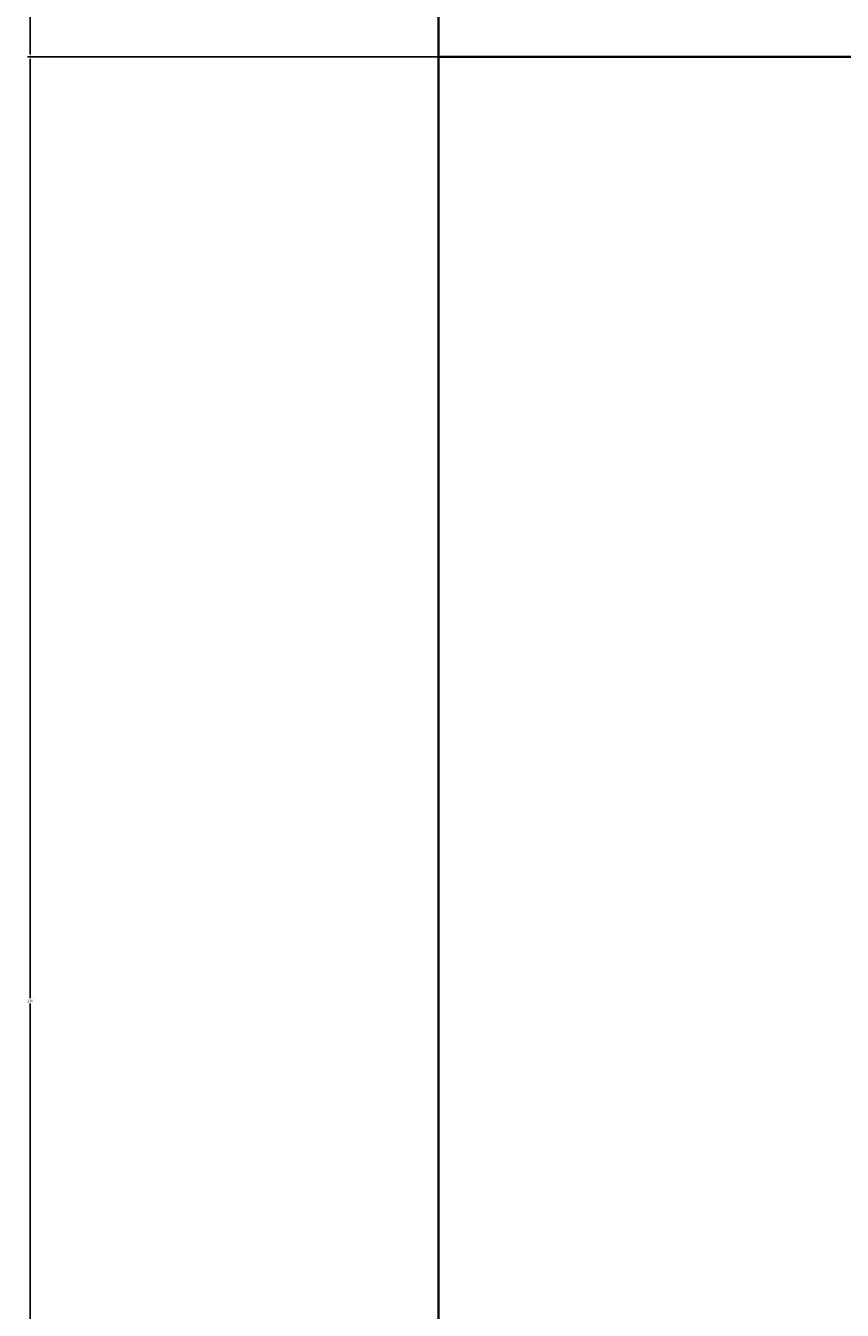
# Model space of a CAD drawing. Units: inches. Extents: x 1911 to 3278, y 2022 to 3108.
# Tile 3 of 13: x 1988 to 2045, y 2178 to 2266. Entities that reach past the tile are written whole.
import ezdxf

# ---------------------------------------------------------------- set-up
doc = ezdxf.new("R2010")
doc.units = ezdxf.units.IN
doc.layers.add('A-ANNO-DIMS', color=2, linetype='Continuous', lineweight=18)
doc.layers.add('A-WALL', color=7, linetype='Continuous', lineweight=35)
doc.styles.get("Standard").update_dxf_attribs({"font": 'arial.ttf'})
doc.dimstyles.get("Standard").update_dxf_attribs({"dimtxt": 0.18, "dimasz": 0.18, "dimexe": 0.18, "dimexo": 0.0625, "dimgap": 0.09, "dimtad": 0, "dimtih": 1, "dimtoh": 1, "dimdec": 4, "dimzin": 0, "dimdsep": 46, "dimtxsty": 'Standard', "dimcen": 0.09, "dimadec": 0, "dimazin": 0, "dimtfac": 1, "dimtdec": 4, "dimtofl": 0, "dimtmove": 0, "dimatfit": 3, "dimfxl": 1, "dimtolj": 1, "dimtzin": 0, "dimarcsym": 0})

# ---------------------------------------------------------------- blocks, each defined once
blk = doc.blocks.new('*D68')
at = {"layer": 'A-ANNO-DIMS', "color": 0, "lineweight": -2, "transparency": 16777216}
for p, q in [((2016.834, 2263.811), (2016.834, 2048.124)), ((2117.834, 2263.811), (2117.834, 2048.124)), ((2017.014, 2048.304), (2067.071, 2048.304)), ((2117.654, 2048.304), (2067.597, 2048.304))]:
    blk.add_line(p, q, dxfattribs=at)
at = {"layer": 'A-ANNO-DIMS', "color": 0, "transparency": 16777216}
for points in [[(2017.014, 2048.334), (2017.014, 2048.274), (2016.834, 2048.304)], [(2117.654, 2048.334), (2117.654, 2048.274), (2117.834, 2048.304)]]:
    blk.add_solid(points, dxfattribs=at)
at = {"layer": 'Defpoints', "color": 0, "transparency": 16777216}
for p in [(2016.834, 2263.873), (2117.834, 2263.873), (2117.834, 2048.304)]:
    blk.add_point(p, dxfattribs=at)
at = {"layer": 'A-ANNO-DIMS', "color": 0, "transparency": 16777216, "insert": (2067.334, 2048.304), "char_height": 0.18, "attachment_point": 5}
blk.add_mtext('\\A1;101', dxfattribs=at)
blk = doc.blocks.new('*D69')
at = {"layer": 'A-ANNO-DIMS', "color": 0, "lineweight": -2, "transparency": 16777216}
for p, q in [((2016.772, 2263.873), (1988.554, 2263.873)), ((1988.734, 2263.693), (1988.734, 2199.055)), ((1988.734, 2134.053), (1988.734, 2198.691)), ((2016.772, 2133.873), (1988.554, 2133.873))]:
    blk.add_line(p, q, dxfattribs=at)
at = {"layer": 'A-ANNO-DIMS', "color": 0, "transparency": 16777216}
for points in [[(1988.704, 2263.693), (1988.764, 2263.693), (1988.734, 2263.873)], [(1988.704, 2134.053), (1988.764, 2134.053), (1988.734, 2133.873)]]:
    blk.add_solid(points, dxfattribs=at)
at = {"layer": 'Defpoints', "color": 0, "transparency": 16777216}
for p in [(2016.834, 2263.873), (1988.734, 2133.873), (2016.834, 2133.873)]:
    blk.add_point(p, dxfattribs=at)
at = {"layer": 'A-ANNO-DIMS', "color": 0, "transparency": 16777216, "insert": (1988.734, 2198.873), "char_height": 0.18, "attachment_point": 5}
blk.add_mtext('\\A1;130', dxfattribs=at)
blk = doc.blocks.new('*D70')
at = {"layer": 'A-ANNO-DIMS', "color": 0, "lineweight": -2, "transparency": 16777216}
for p, q in [((2134.103, 2181.811), (2134.103, 2048.124)), ((2016.834, 2133.811), (2016.834, 2048.124)), ((2017.014, 2048.304), (2075.014, 2048.304)), ((2133.923, 2048.304), (2075.924, 2048.304))]:
    blk.add_line(p, q, dxfattribs=at)
at = {"layer": 'A-ANNO-DIMS', "color": 0, "transparency": 16777216}
for points in [[(2017.014, 2048.334), (2017.014, 2048.274), (2016.834, 2048.304)], [(2133.923, 2048.334), (2133.923, 2048.274), (2134.103, 2048.304)]]:
    blk.add_solid(points, dxfattribs=at)
at = {"layer": 'Defpoints', "color": 0, "transparency": 16777216}
for p in [(2134.103, 2181.873), (2016.834, 2133.873), (2134.103, 2048.304)]:
    blk.add_point(p, dxfattribs=at)
at = {"layer": 'A-ANNO-DIMS', "color": 0, "transparency": 16777216, "insert": (2075.469, 2048.304), "char_height": 0.18, "attachment_point": 5}
blk.add_mtext('\\A1;117.27', dxfattribs=at)
blk = doc.blocks.new('*D72')
at = {"layer": 'A-ANNO-DIMS', "color": 0, "lineweight": -2, "transparency": 16777216}
for p, q in [((2016.772, 2358.3), (1988.554, 2358.3)), ((1988.734, 2358.12), (1988.734, 2311.269)), ((1988.734, 2264.053), (1988.734, 2310.905)), ((2016.772, 2263.873), (1988.554, 2263.873))]:
    blk.add_line(p, q, dxfattribs=at)
at = {"layer": 'A-ANNO-DIMS', "color": 0, "transparency": 16777216}
for points in [[(1988.704, 2358.12), (1988.764, 2358.12), (1988.734, 2358.3)], [(1988.704, 2264.053), (1988.764, 2264.053), (1988.734, 2263.873)]]:
    blk.add_solid(points, dxfattribs=at)
at = {"layer": 'Defpoints', "color": 0, "transparency": 16777216}
for p in [(1988.734, 2358.3), (2016.834, 2358.3), (2016.834, 2263.873)]:
    blk.add_point(p, dxfattribs=at)
at = {"layer": 'A-ANNO-DIMS', "color": 0, "transparency": 16777216, "insert": (1988.734, 2311.087), "char_height": 0.18, "attachment_point": 5}
blk.add_mtext('\\A1;94.43', dxfattribs=at)

msp = doc.modelspace()

# ---------------------------------------------------------------- linework, layer by layer
at = {"layer": 'A-WALL'}
for p, q in [((2016.8344, 2620.8733), (2016.8344, 2133.8733)), ((2016.8344, 2620.8733), (2016.8344, 2133.8733)), ((2016.8344, 2263.8733), (2117.8344, 2263.8733))]:
    msp.add_line(p, q, dxfattribs=at)

# ---------------------------------------------------------------- dimensions: what is measured, and where the dimension line sits
at = {"layer": 'A-ANNO-DIMS'}
for base, p2, override, picture, middle in [((1988.7344, 2358.3003), (2016.8344, 2358.3003), {"dimdec": 2, "dimlfac": 1, "dimrnd": 0, "dimzin": 0, "dimdsep": 46, "dimlunit": 2}, '*D72', (1988.7344, 2311.0868)), ((1988.7344, 2133.8733), (2016.8344, 2133.8733), {"dimdec": 0, "dimlfac": 1, "dimrnd": 0, "dimzin": 0, "dimdsep": 46, "dimlunit": 2}, '*D69', (1988.7344, 2198.8733))]:
    dim = msp.add_linear_dim(base=base, p1=(2016.8344, 2263.8733), p2=p2, angle=90, dimstyle='Standard', override=override, dxfattribs=at)
    dim.commit()
    dim.dimension.update_dxf_attribs({"geometry": picture, "text_midpoint": middle})
for base, p1, p2, override, picture, middle in [((2117.8344, 2048.3043), (2016.8344, 2263.8733), (2117.8344, 2263.8733), {"dimdec": 0, "dimlfac": 1, "dimrnd": 0, "dimzin": 0, "dimdsep": 46, "dimlunit": 2}, '*D68', (2067.3344, 2048.3043)), ((2134.1034, 2048.3043), (2016.8344, 2133.8733), (2134.1034, 2181.8733), {"dimdec": 2, "dimlfac": 1, "dimrnd": 0, "dimzin": 0, "dimdsep": 46, "dimlunit": 2}, '*D70', (2075.4689, 2048.3043))]:
    dim = msp.add_linear_dim(base=base, p1=p1, p2=p2, dimstyle='Standard', override=override, dxfattribs=at)
    dim.commit()
    dim.dimension.update_dxf_attribs({"geometry": picture, "text_midpoint": middle})

doc.saveas('drawing.dxf')
